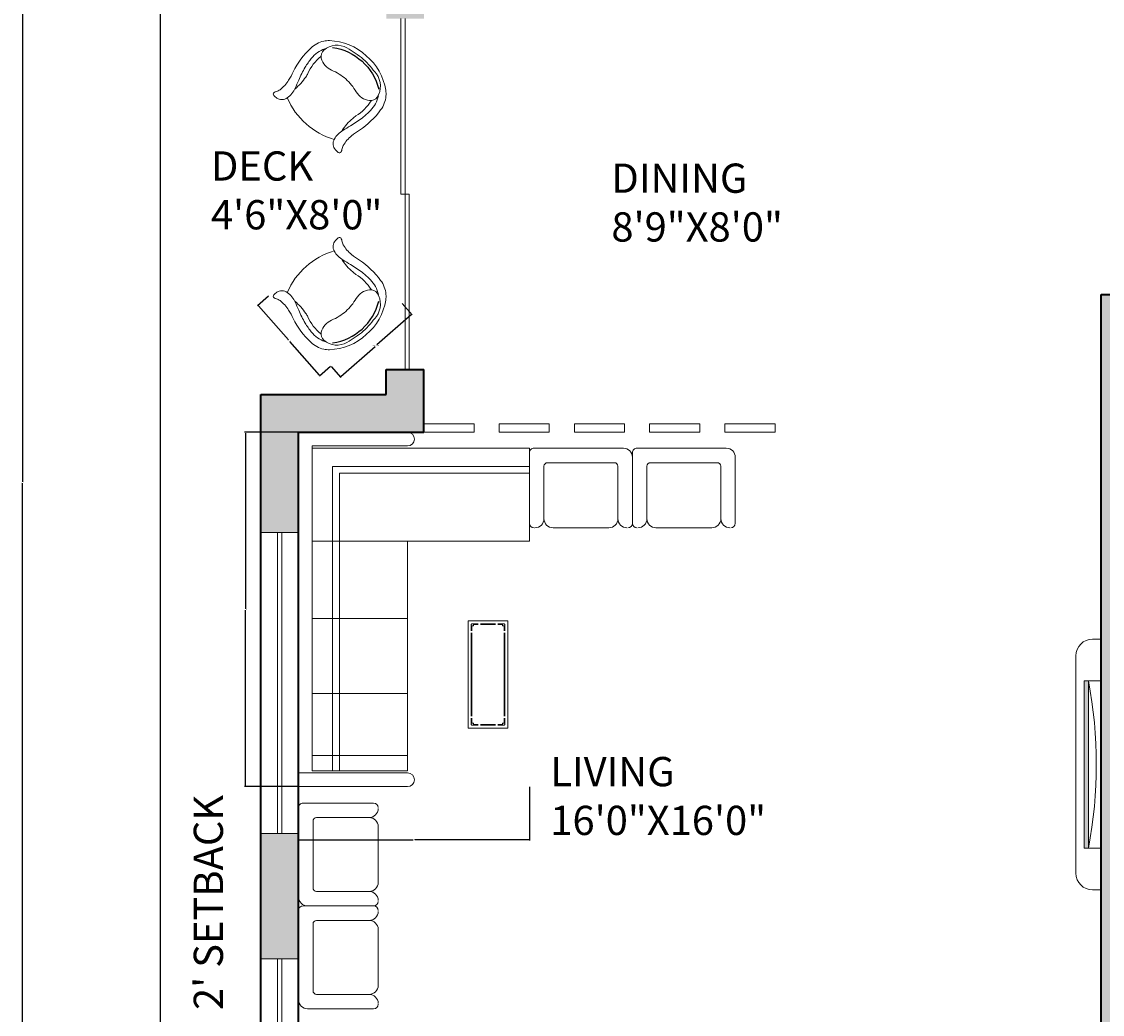
# Model space of a CAD drawing. Units: inches. Extents: x 3386 to 4477, y 1118 to 1824.
# Tile 2 of 7: x 3386 to 3645, y 1364 to 1601. Entities that reach past the tile are written whole.
import ezdxf

# ---------------------------------------------------------------- set-up
doc = ezdxf.new("R2010")
doc.units = ezdxf.units.IN
for name, color, linetype, lineweight in [('A-ANNO-DIMS', 2, 'Continuous', 18), ('A-ANNO-TEXT', 7, 'Continuous', 18), ('A-AREA-IDEN', 7, 'Continuous', 18), ('A-DOOR', 4, 'Continuous', 18), ('A-EQPM', 9, 'Continuous', 18), ('A-FLOR-SCRN', 7, 'Continuous', 18), ('A-FURN', 8, 'Continuous', 18), ('A-GLAZ', 4, 'Continuous', 18), ('A-WALL', 7, 'Continuous', 35), ('C-PROP', 7, 'Continuous', 25)]:
    doc.layers.add(name, color=color, linetype=linetype, lineweight=lineweight)
doc.layers.add('A-EQPM-PATT', color=18, linetype='Continuous', lineweight=13, true_color=0x000000)
doc.layers.add('A-WALL-PATT', color=18, linetype='Continuous', lineweight=13, true_color=0x000000)
doc.layers.add('IFF-FURN-DETAIL', color=250, linetype='Continuous')
doc.styles.get("Standard").update_dxf_attribs({"font": 'arial.ttf'})
doc.dimstyles.get("Standard").update_dxf_attribs({"dimtxt": 0.18, "dimasz": 0.18, "dimexe": 0.18, "dimexo": 0.0625, "dimgap": 0.09, "dimtad": 0, "dimtih": 1, "dimtoh": 1, "dimdec": 4, "dimzin": 0, "dimdsep": 46, "dimtxsty": 'Standard', "dimcen": 0.09, "dimadec": 0, "dimazin": 0, "dimtfac": 1, "dimtdec": 4, "dimtofl": 0, "dimtmove": 0, "dimatfit": 3, "dimfxl": 1, "dimtolj": 1, "dimtzin": 0, "dimarcsym": 0})

# ---------------------------------------------------------------- blocks, each defined once
blk = doc.blocks.new('sofa-27')
at = {"color": 0, "linetype": 'ByBlock'}
for p, q in [((0.0945, 0.5198), (0.459, 0.5198)), ((-0.0591, 0.0591), (-0.0591, 0.4902)), ((0.0354, 0.1181), (0.0354, 0.4607)), ((0.518, 0.1181), (0.518, 0.4607)), ((0.6125, 0.0295), (0.6125, 0.4902)), ((0.4944, 0.0945), (0.0591, 0.0945)), ((0.583, 0), (0, 0))]:
    blk.add_line(p, q, dxfattribs=at)
for centre, radius, start, end in [((-0.0295, 0.4902), 0.0295, 90, 180), ((-0.0236, 0.4607), 0.0591, 360, 90), ((0.0945, 0.4607), 0.0591, 90, 180), ((0.459, 0.4607), 0.0591, 0, 90), ((0.5771, 0.4607), 0.0591, 90, 180), ((0.583, 0.4902), 0.0295, 0, 90), ((0.0591, 0.1181), 0.0236, 180, 270), ((0.4944, 0.1181), 0.0236, 270, 0), ((0, 0.0591), 0.0591, 180, 270), ((0.583, 0.0295), 0.0295, 270, 0)]:
    blk.add_arc(centre, radius, start, end, dxfattribs=at)
blk = doc.blocks.new('TABLE-30A')
at = {"color": 0, "linetype": 'ByBlock'}
for p, q in [((0, 0), (0, 0.55)), ((0, 0.55), (1.5, 0.55)), ((0.051, 0.508), (0.042, 0.499)), ((0.042, 0.499), (0.042, 0.478)), ((0.042, 0.478), (0.072, 0.478)), ((0.042, 0.478), (0.042, 0.41)), ((0.072, 0.508), (0.051, 0.508)), ((0.051, 0.478), (0.051, 0.41)), ((0.072, 0.478), (0.072, 0.508)), ((0.072, 0.508), (0.14, 0.508)), ((0.072, 0.499), (0.14, 0.499)), ((1.331, 0.508), (0.169, 0.508)), ((1.331, 0.499), (0.169, 0.499)), ((1.428, 0.508), (1.36, 0.508)), ((1.428, 0.499), (1.36, 0.499)), ((1.428, 0.508), (1.428, 0.478)), ((1.449, 0.508), (1.428, 0.508)), ((1.428, 0.478), (1.458, 0.478)), ((1.458, 0.499), (1.449, 0.508)), ((1.449, 0.478), (1.449, 0.41)), ((1.458, 0.478), (1.458, 0.499)), ((1.458, 0.478), (1.458, 0.41)), ((1.5, 0.55), (1.5, 0)), ((0.042, 0.169), (0.042, 0.381)), ((0.051, 0.169), (0.051, 0.381)), ((1.449, 0.381), (1.449, 0.169)), ((1.458, 0.381), (1.458, 0.169)), ((1.5, 0), (0, 0)), ((0.042, 0.072), (0.042, 0.14)), ((0.042, 0.072), (0.042, 0.051)), ((0.072, 0.072), (0.042, 0.072)), ((0.042, 0.051), (0.051, 0.042)), ((0.051, 0.072), (0.051, 0.14)), ((0.051, 0.042), (0.072, 0.042)), ((0.072, 0.042), (0.072, 0.072)), ((0.072, 0.051), (0.14, 0.051)), ((0.072, 0.042), (0.14, 0.042)), ((0.169, 0.051), (1.331, 0.051)), ((0.169, 0.042), (1.331, 0.042)), ((1.428, 0.051), (1.36, 0.051)), ((1.428, 0.042), (1.36, 0.042)), ((1.428, 0.072), (1.428, 0.042)), ((1.458, 0.072), (1.428, 0.072)), ((1.428, 0.042), (1.449, 0.042)), ((1.449, 0.072), (1.449, 0.14)), ((1.449, 0.042), (1.458, 0.051)), ((1.458, 0.072), (1.458, 0.14)), ((1.458, 0.051), (1.458, 0.072))]:
    blk.add_line(p, q, dxfattribs=at)
blk = doc.blocks.new('12')
at = {"color": 0}
for p, q in [((5656.26, 3021.25), (5553.9, 3021.25)), ((5553.9, 3021.25), (5553.9, 2989.76)), ((5557.83, 3021.25), (5557.83, 2989.76)), ((5656.26, 2989.76), (5656.26, 3021.25)), ((5652.32, 3017.31), (5558.49, 3017.31)), ((5558.49, 3017.31), (5558.49, 2989.76)), ((5562.89, 3017.31), (5562.89, 2989.76)), ((5580.8, 3017.31), (5580.8, 2989.76)), ((5602.45, 3017.31), (5602.45, 2989.76)), ((5624.76, 3017.31), (5624.76, 2954.53)), ((5651.66, 3017.31), (5651.66, 2954.53)), ((5652.32, 2989.76), (5652.32, 3017.31)), ((5646.42, 3011.41), (5558.49, 3011.41)), ((5646.42, 2954.53), (5646.42, 3011.41)), ((5644.45, 3009.44), (5558.49, 3009.44)), ((5644.45, 2954.53), (5644.45, 3009.44)), ((5624.76, 2995), (5624.76, 2954.53)), ((5558.49, 2989.76), (5624.76, 2989.76)), ((5651.66, 2954.53), (5624.76, 2954.53))]:
    blk.add_line(p, q, dxfattribs=at)
for centre in [(5555.86, 2989.76), (5654.29, 2989.76)]:
    blk.add_arc(centre, 1.97, 180, 0, dxfattribs=at)
at = {"xscale": -20.70834898381633, "yscale": 20.70834898381633, "zscale": 20.70834898381633}
blk.add_blockref('TABLE-30A', (5601.8, 2960.82), dxfattribs=at)
blk = doc.blocks.new('ILNG95')
for points in [[(120, 308, -0.32971), (51, 384, -0.036099), (50, 422, -0.497733), (75, 439, -0.070621), (96, 429, 0.101868), (133, 414, 0.091794), (259, 412, 0.024114), (351, 433, -0.090294), (638, 458, -0.132412), (775, 407, -0.068618), (816, 368, -0.184346), (943, 0, 1.803905)], [(120, 308, 0.138132), (244, 313, 0.001085), (325, 339, -0.034227), (462, 375, -0.033255), (567, 387, -0.137428), (727, 350, -4.561553)], [(120, 308, 0.138132), (244, 313, 0.001085), (325, 339, -0.034227), (462, 375, -0.033255), (567, 387, -0.137428), (727, 350, -4.561553)], [(235, 308, 0.064243), (394, 307, 0.04414), (433, 315, -0.118032), (643, 329, -6.296816)], [(235, 308, 0.064243), (394, 307, 0.04414), (433, 315, -0.118032), (643, 329, -6.296816)], [(639, 0, 0.078302), (612, 161, -0.233633), (633, 315, -0.28763), (710, 349, -0.317923), (875, 193, -0.032882), (900, 0, 1.140397)], [(639, 0, 0.078302), (612, 161, -0.233633), (633, 315, -0.28763), (710, 349, -0.317923), (875, 193, -0.032882), (900, 0, 1.140397)], [(120, -308, 0.32971), (51, -384, 0.036099), (50, -422, 0.497733), (75, -439, 0.070621), (96, -429, -0.101868), (133, -414, -0.091794), (259, -412, -0.024114), (351, -433, 0.090294), (638, -458, 0.132412), (775, -407, 0.068618), (816, -368, 0.184346), (943, 0, -1.803905)], [(639, 0, -0.078302), (612, -161, 0.233633), (633, -315, 0.28763), (710, -349, 0.317923), (875, -193, 0.032882), (900, 0, -1.140397)], [(639, 0, -0.078302), (612, -161, 0.233633), (633, -315, 0.28763), (710, -349, 0.317923), (875, -193, 0.032882), (900, 0, -1.140397)], [(120, -308, -0.138132), (244, -313, -0.001085), (325, -339, 0.034227), (462, -375, 0.033255), (567, -387, 0.137428), (727, -350, 4.561553)], [(120, -308, -0.138132), (244, -313, -0.001085), (325, -339, 0.034227), (462, -375, 0.033255), (567, -387, 0.137428), (727, -350, 4.561553)], [(235, -308, -0.064243), (394, -307, -0.04414), (433, -315, 0.118032), (643, -329, 6.296816)], [(235, -308, -0.064243), (394, -307, -0.04414), (433, -315, 0.118032), (643, -329, 6.296816)]]:
    blk.add_lwpolyline(points, format="xyb")
blk.add_arc((759, 1), 709, 154.3281, 205.801)
at = {"layer": 'IFF-FURN-DETAIL'}
blk.add_arc((326, -2), 549, 326.8997, 34.6691, dxfattribs=at)
blk.add_arc((326, -2), 549, 326.8997, 34.6691, dxfattribs=at)
blk = doc.blocks.new('WIN-48IN')
for p, q in [((0, 48), (9, 48)), ((4, 0), (4, 48)), ((5, 0), (5, 48)), ((0, 0), (9, 0))]:
    blk.add_line(p, q)
blk = doc.blocks.new('WIN-72IN')
for p, q in [((0, 0), (0, 9)), ((72, 0), (72, 9)), ((0, 5), (72, 5)), ((0, 4), (72, 4))]:
    blk.add_line(p, q)
blk = doc.blocks.new('DOOR-SLIDING-84IN')
for p, q in [((0, 42), (0, 84)), ((1, 84), (1, 0)), ((1, 42), (0, 42)), ((1, 42), (2, 42)), ((2, 42), (2, 0))]:
    blk.add_line(p, q)
blk = doc.blocks.new('SCREEN-LIVING-DINING')
for points in [[(0, 0), (12, 0), (12, 2), (0, 2)], [(18, 0), (30, 0), (30, 2), (18, 2)], [(36, 0), (48, 0), (48, 2), (36, 2)], [(54, 0), (66, 0), (66, 2), (54, 2)], [(72, 0), (84, 0), (84, 2), (72, 2)]]:
    blk.add_lwpolyline(points, close=True)
blk = doc.blocks.new('*D73')
at = {"layer": 'A-ANNO-DIMS', "color": 0, "lineweight": -2, "transparency": 16777216}
for p, q in [((3477.49, 1533.65), (3479.83, 1531)), ((3479.57, 1531.01), (3471.39, 1523.79)), ((3462.78, 1516.21), (3470.97, 1523.43)), ((3460.43, 1518.6), (3462.77, 1515.95))]:
    blk.add_line(p, q, dxfattribs=at)
at = {"layer": 'A-ANNO-DIMS', "color": 0, "transparency": 16777216}
for points in [[(3479.55, 1531.04), (3479.59, 1530.99), (3479.71, 1531.13)], [(3462.76, 1516.23), (3462.8, 1516.18), (3462.65, 1516.09)]]:
    blk.add_solid(points, dxfattribs=at)
at = {"layer": 'Defpoints', "color": 0, "transparency": 16777216}
for p in [(3477.45, 1533.69), (3479.71, 1531.13), (3460.39, 1518.65)]:
    blk.add_point(p, dxfattribs=at)
at = {"layer": 'A-ANNO-DIMS', "color": 0, "transparency": 16777216, "insert": (3471.18, 1523.61), "char_height": 0.18, "attachment_point": 5}
blk.add_mtext('\\A1;CHAIR 23 TYP.', dxfattribs=at)
blk = doc.blocks.new('*D74')
at = {"layer": 'A-ANNO-DIMS', "color": 0, "lineweight": -2, "transparency": 16777216}
for p, q in [((3445.5, 1535.44), (3442.85, 1533.1)), ((3443.11, 1533.09), (3450.25, 1524.99)), ((3457.71, 1516.52), (3450.57, 1524.62)), ((3460.34, 1518.6), (3457.7, 1516.27))]:
    blk.add_line(p, q, dxfattribs=at)
at = {"layer": 'A-ANNO-DIMS', "color": 0, "transparency": 16777216}
for points in [[(3443.13, 1533.11), (3443.08, 1533.07), (3442.99, 1533.22)], [(3457.74, 1516.54), (3457.69, 1516.5), (3457.83, 1516.39)]]:
    blk.add_solid(points, dxfattribs=at)
at = {"layer": 'Defpoints', "color": 0, "transparency": 16777216}
for p in [(3445.55, 1535.48), (3460.39, 1518.65), (3457.83, 1516.39)]:
    blk.add_point(p, dxfattribs=at)
at = {"layer": 'A-ANNO-DIMS', "color": 0, "transparency": 16777216, "insert": (3450.41, 1524.81), "char_height": 0.18, "attachment_point": 5}
blk.add_mtext('\\A1;22 TYP.', dxfattribs=at)
blk = doc.blocks.new('*D91')
at = {"layer": 'A-ANNO-DIMS', "color": 0, "lineweight": -2, "transparency": 16777216}
for p, q in [((3452.59, 1502.87), (3439.76, 1502.87)), ((3439.94, 1502.69), (3439.94, 1460.66)), ((3439.94, 1418.27), (3439.94, 1460.3)), ((3452.59, 1418.09), (3439.76, 1418.09))]:
    blk.add_line(p, q, dxfattribs=at)
at = {"layer": 'A-ANNO-DIMS', "color": 0, "transparency": 16777216}
for points in [[(3439.91, 1502.69), (3439.97, 1502.69), (3439.94, 1502.87)], [(3439.91, 1418.27), (3439.97, 1418.27), (3439.94, 1418.09)]]:
    blk.add_solid(points, dxfattribs=at)
at = {"layer": 'Defpoints', "color": 0, "transparency": 16777216}
for p in [(3439.94, 1502.87), (3452.66, 1502.87), (3452.66, 1418.09)]:
    blk.add_point(p, dxfattribs=at)
at = {"layer": 'A-ANNO-DIMS', "color": 0, "transparency": 16777216, "insert": (3439.94, 1460.48), "char_height": 0.18, "attachment_point": 5}
blk.add_mtext('\\A1;L-SOFA 85', dxfattribs=at)
blk = doc.blocks.new('*D92')
at = {"layer": 'A-ANNO-DIMS', "color": 0, "lineweight": -2, "transparency": 16777216}
for p, q in [((3452.66, 1418.03), (3452.66, 1405.19)), ((3507.92, 1418.03), (3507.92, 1405.19)), ((3452.84, 1405.37), (3480.07, 1405.37)), ((3507.74, 1405.37), (3480.51, 1405.37))]:
    blk.add_line(p, q, dxfattribs=at)
at = {"layer": 'A-ANNO-DIMS', "color": 0, "transparency": 16777216}
for points in [[(3452.84, 1405.4), (3452.84, 1405.34), (3452.66, 1405.37)], [(3507.74, 1405.4), (3507.74, 1405.34), (3507.92, 1405.37)]]:
    blk.add_solid(points, dxfattribs=at)
at = {"layer": 'Defpoints', "color": 0, "transparency": 16777216}
for p in [(3452.66, 1418.09), (3507.92, 1418.09), (3452.66, 1405.37)]:
    blk.add_point(p, dxfattribs=at)
at = {"layer": 'A-ANNO-DIMS', "color": 0, "transparency": 16777216, "insert": (3480.29, 1405.37), "char_height": 0.18, "attachment_point": 5}
blk.add_mtext('\\A1;55', dxfattribs=at)
blk = doc.blocks.new('*D102')
at = {"layer": 'A-ANNO-DIMS', "color": 0, "lineweight": -2, "transparency": 16777216}
for p, q in [((3419.59, 1790.87), (3386.43, 1790.87)), ((3386.61, 1790.69), (3386.61, 1491.05)), ((3386.61, 1191.05), (3386.61, 1490.69)), ((3419.59, 1190.87), (3386.43, 1190.87))]:
    blk.add_line(p, q, dxfattribs=at)
at = {"layer": 'A-ANNO-DIMS', "color": 0, "transparency": 16777216}
for points in [[(3386.58, 1790.69), (3386.64, 1790.69), (3386.61, 1790.87)], [(3386.58, 1191.05), (3386.64, 1191.05), (3386.61, 1190.87)]]:
    blk.add_solid(points, dxfattribs=at)
at = {"layer": 'Defpoints', "color": 0, "transparency": 16777216}
for p in [(3386.61, 1790.87), (3419.66, 1790.87), (3419.66, 1190.87)]:
    blk.add_point(p, dxfattribs=at)
at = {"layer": 'A-ANNO-DIMS', "color": 0, "transparency": 16777216, "insert": (3386.61, 1490.87), "char_height": 0.18, "attachment_point": 5}
blk.add_mtext('\\A1;600', dxfattribs=at)

msp = doc.modelspace()

# ---------------------------------------------------------------- hatches: boundary and pattern name
at = {"layer": 'A-EQPM-PATT'}
h = msp.add_hatch(color=256, dxfattribs=at)
h.dxf.hatch_style = 1
h.paths.add_polyline_path([(3640.66, 1403.37), (3641.66, 1403.37), (3641.66, 1443.37), (3640.66, 1443.37)])
at = {"layer": 'A-WALL-PATT'}
h = msp.add_hatch(color=256, dxfattribs=at)
h.dxf.hatch_style = 1
h.paths.add_polyline_path([(3443.66, 1221.87), (3452.66, 1221.87), (3452.66, 1301.87), (3458.66, 1301.87), (3458.66, 1310.87), (3452.66, 1310.87), (3452.66, 1328.87), (3443.66, 1328.87)])
h.paths.add_polyline_path([(3506.66, 1310.87), (3506.66, 1306.37), (3506.66, 1301.87), (3530.66, 1301.87), (3530.66, 1310.87)])
h.paths.add_polyline_path([(3653.66, 1301.87), (3653.66, 1382.87), (3662.66, 1382.87), (3662.66, 1391.87), (3653.66, 1391.87), (3653.66, 1529.87), (3659.66, 1529.87), (3659.66, 1535.87), (3644.66, 1535.87), (3644.66, 1310.87), (3602.66, 1310.87), (3602.66, 1301.87)])
h.paths.add_polyline_path([(3452.66, 1406.87), (3443.66, 1406.87), (3443.66, 1376.87), (3452.66, 1376.87), (3452.66, 1388.44)])
h.paths.add_polyline_path([(3452.66, 1478.87), (3452.66, 1502.87), (3478.74, 1502.87), (3482.66, 1502.87), (3482.66, 1504.87), (3482.66, 1517.87), (3473.66, 1517.87), (3473.66, 1511.87), (3443.66, 1511.87), (3443.66, 1478.87)])
h.paths.add_polyline_path([(3773.66, 1391.87), (3710.66, 1391.87), (3710.66, 1382.87), (3773.66, 1382.87)], flags=17)
h.paths.add_polyline_path([(3824.66, 1391.87), (3806.66, 1391.87), (3806.66, 1469.87), (3809.66, 1469.87), (3809.66, 1472.87), (3809.66, 1475.87), (3806.66, 1475.87), (3806.66, 1478.87), (3800.66, 1478.87), (3800.66, 1463.32), (3800.66, 1391.87), (3797.66, 1391.87), (3797.66, 1382.87), (3824.66, 1382.87)], flags=17)
h.paths.add_polyline_path([(3866.66, 1469.87), (3866.66, 1391.87), (3848.66, 1391.87), (3848.66, 1382.87), (3875.66, 1382.87), (3875.66, 1547.87), (3866.66, 1547.87), (3866.66, 1535.87), (3695.66, 1535.87), (3695.66, 1529.87), (3800.66, 1529.87), (3800.66, 1508.87), (3806.66, 1508.87), (3806.66, 1529.87), (3866.66, 1529.87), (3866.66, 1475.87), (3839.66, 1475.87), (3839.66, 1469.87)])
h.paths.add_polyline_path([(3875.66, 1673.87), (3866.66, 1673.87), (3866.66, 1663.37), (3866.66, 1647.44), (3866.66, 1613.87), (3761.66, 1613.87), (3761.66, 1607.87), (3866.66, 1607.87), (3866.66, 1595.87), (3875.66, 1595.87)])
h.paths.add_polyline_path([(3473.66, 1607.87), (3473.66, 1601.87), (3482.66, 1601.87), (3482.66, 1616.87), (3452.66, 1616.87), (3452.66, 1640.87), (3443.66, 1640.87), (3443.66, 1607.87)])
h.paths.add_polyline_path([(3491.66, 1736.87), (3491.66, 1745.87), (3478.95, 1745.87), (3443.66, 1745.87), (3443.66, 1688.87), (3452.66, 1688.87), (3452.66, 1736.87)])
h.paths.add_polyline_path([(3551.66, 1745.87), (3539.66, 1745.87), (3539.66, 1736.87), (3551.66, 1736.87)])
h.paths.add_polyline_path([(3587.66, 1745.87), (3581.66, 1745.87), (3581.66, 1741.37), (3581.66, 1736.87), (3587.66, 1736.87), (3587.66, 1712.87), (3596.66, 1712.87), (3596.66, 1757.87), (3644.66, 1757.87), (3644.66, 1679.87), (3596.66, 1679.87), (3596.66, 1682.87), (3592.16, 1682.87), (3587.66, 1682.87), (3587.66, 1607.87), (3602.66, 1607.87), (3602.66, 1613.87), (3596.66, 1613.87), (3596.66, 1673.87), (3644.66, 1673.87), (3644.66, 1613.87), (3638.66, 1613.87), (3638.66, 1610.87), (3638.66, 1607.87), (3725.66, 1607.87), (3725.66, 1613.87), (3722.66, 1613.87), (3722.66, 1634.87), (3716.66, 1634.87), (3716.66, 1613.87), (3650.66, 1613.87), (3650.66, 1673.87), (3683.66, 1673.87), (3683.66, 1679.87), (3650.66, 1679.87), (3650.66, 1757.87), (3671.66, 1757.87), (3671.66, 1766.87), (3587.66, 1766.87)])
h.paths.add_polyline_path([(3716.66, 1757.87), (3716.66, 1679.87), (3713.66, 1679.87), (3713.66, 1673.87), (3716.66, 1673.87), (3716.66, 1664.87), (3722.66, 1664.87), (3722.66, 1757.87), (3728.66, 1757.87), (3728.66, 1766.87), (3695.66, 1766.87), (3695.66, 1757.87)])
h.paths.add_polyline_path([(3806.66, 1757.87), (3806.66, 1766.87), (3776.66, 1766.87), (3776.66, 1757.87)])
h.paths.add_polyline_path([(3875.66, 1766.87), (3854.66, 1766.87), (3854.66, 1757.87), (3866.66, 1757.87), (3866.66, 1733.87), (3875.66, 1733.87)])

# ---------------------------------------------------------------- linework, layer by layer
at = {"layer": 'A-EQPM'}
for p, q in [((3644.66, 1453.37), (3642.66, 1453.37)), ((3644.66, 1393.37), (3644.66, 1453.37)), ((3638.66, 1449.37), (3638.66, 1397.37)), ((3644.66, 1443.37), (3640.66, 1443.37)), ((3640.66, 1403.37), (3640.66, 1443.37)), ((3641.66, 1403.37), (3641.66, 1443.37)), ((3644.66, 1403.37), (3640.66, 1403.37)), ((3644.66, 1393.37), (3642.66, 1393.37))]:
    msp.add_line(p, q, dxfattribs=at)
for centre, radius, start, end in [((3642.66, 1449.37), 4, 90, 180), ((3536.62, 1423.37), 106.92, 349.2189, 10.7811), ((3642.66, 1397.37), 4, 180, 270)]:
    msp.add_arc(centre, radius, start, end, dxfattribs=at)
at = {"layer": 'A-WALL'}
for p, q in [((3644.66, 1310.87), (3644.66, 1535.87)), ((3644.66, 1535.87), (3659.66, 1535.87)), ((3473.66, 1511.87), (3473.66, 1517.87)), ((3473.66, 1517.87), (3482.66, 1517.87)), ((3482.66, 1502.87), (3482.66, 1517.87)), ((3443.66, 1221.87), (3443.66, 1511.87)), ((3443.66, 1511.87), (3473.66, 1511.87)), ((3452.66, 1502.87), (3482.66, 1502.87)), ((3452.66, 1310.87), (3452.66, 1502.87))]:
    msp.add_line(p, q, dxfattribs=at)
at = {"layer": 'C-PROP'}
msp.add_lwpolyline([(3419.66, 1790.87), (3899.66, 1790.87), (3899.66, 1190.87), (3419.66, 1190.87)], close=True, dxfattribs=at)

# ---------------------------------------------------------------- block references
at = {"layer": 'A-DOOR'}
msp.add_blockref('DOOR-SLIDING-84IN', (3477.16, 1517.87), dxfattribs=at)
at = {"layer": 'A-FLOR-SCRN'}
msp.add_blockref('SCREEN-LIVING-DINING', (3482.66, 1502.87), dxfattribs=at)
at = {"layer": 'A-FURN'}
for name, p, xscale, yscale, zscale, rotation in [('ILNG95', (3453.65, 1575.73), -0.0243705291132055, 0.0243705291132055, 0.0243705291132055, 228.5881218623716), ('ILNG95', (3453.65, 1543.48), 0.0243705291132055, 0.0243705291132055, 0.0243705291132055, 311.4118781376284), ('12', (5954.88, -3181.69), 0.8282073146500575, 0.8282073146500575, 0.8282073146500575, 90.00000000000003), ('sofa-27', (3530.38, 1499.06), 36.66436083614781, 36.66436083614781, 36.66436083614781, 180), ('sofa-27', (3555, 1499.06), 36.66436083614781, 36.66436083614781, 36.66436083614781, 180), ('sofa-27', (3452.66, 1391.69), -36.66436083614781, 36.66436083614781, 36.66436083614781, 269.9999999999598), ('sofa-27', (3452.66, 1367.07), -36.66436083614781, 36.66436083614781, 36.66436083614781, 269.9999999999598)]:
    msp.add_blockref(name, p, dxfattribs=dict(at, xscale=xscale, yscale=yscale, zscale=zscale, rotation=rotation))
at = {"layer": 'A-GLAZ'}
for name, p, rotation in [('WIN-72IN', (3443.66, 1478.87), 270.0000000000004), ('WIN-48IN', (3452.66, 1376.87), 180)]:
    msp.add_blockref(name, p, dxfattribs=dict(at, rotation=rotation))

# ---------------------------------------------------------------- texts
at = {"layer": 'A-ANNO-TEXT', "insert": (3427.58, 1364.63), "char_height": 7, "attachment_point": 1, "rotation": 90}
msp.add_mtext_dynamic_manual_height_columns("{\\fTimes New Roman|b0|i0|c0|p18;2' SETBACK}", width=79.5604, gutter_width=12.5, heights=[0], dxfattribs=at)
at = {"layer": 'A-AREA-IDEN', "char_height": 7, "attachment_point": 1}
for s, insert in [('{\\fTimes New Roman|b0|i0|c0|p18;DECK\\P4\'6"X8\'0"}', (3431.7, 1570.09)), ('{\\fTimes New Roman|b0|i0|c0|p18;DINING\\P8\'9"X8\'0"}', (3527.51, 1567.17)), ('{\\fTimes New Roman|b0|i0|c0|p18;LIVING\\P16\'0"X16\'0"}', (3512.9, 1425.17))]:
    msp.add_mtext_dynamic_manual_height_columns(s, width=79.5604, gutter_width=12.5, heights=[0], dxfattribs=dict(at, insert=insert))

# ---------------------------------------------------------------- dimensions: what is measured, and where the dimension line sits
at = {"layer": 'A-ANNO-DIMS'}
for base, p1, p2, angle, picture, middle in [((3386.61, 1790.87), (3419.66, 1190.87), (3419.66, 1790.87), 90, '*D102', (3386.61, 1490.87)), ((3452.66, 1405.37), (3507.92, 1418.09), (3452.66, 1418.09), 180, '*D92', (3480.29, 1405.37))]:
    dim = msp.add_linear_dim(base=base, p1=p1, p2=p2, angle=angle, dimstyle='Standard', override={"dimdec": 0, "dimlfac": 1, "dimrnd": 0, "dimzin": 0, "dimdsep": 46, "dimlunit": 2}, dxfattribs=at)
    dim.commit()
    dim.dimension.update_dxf_attribs({"geometry": picture, "text_midpoint": middle})
for base, p1, p2, angle, text, picture, middle in [((3457.83, 1516.39), (3445.55, 1535.48), (3460.39, 1518.65), 311.4119, '<> TYP.', '*D74', (3450.41, 1524.81)), ((3479.71, 1531.13), (3460.39, 1518.65), (3477.45, 1533.69), 41.4119, 'CHAIR <> TYP.', '*D73', (3471.18, 1523.61)), ((3439.94, 1502.87), (3452.66, 1418.09), (3452.66, 1502.87), 90, 'L-SOFA <>', '*D91', (3439.94, 1460.48))]:
    dim = msp.add_linear_dim(base=base, p1=p1, p2=p2, angle=angle, text=text, dimstyle='Standard', override={"dimdec": 0, "dimlfac": 1, "dimrnd": 0, "dimzin": 0, "dimdsep": 46, "dimlunit": 2}, dxfattribs=at)
    dim.commit()
    dim.dimension.update_dxf_attribs({"geometry": picture, "text_midpoint": middle})

doc.saveas('drawing.dxf')
